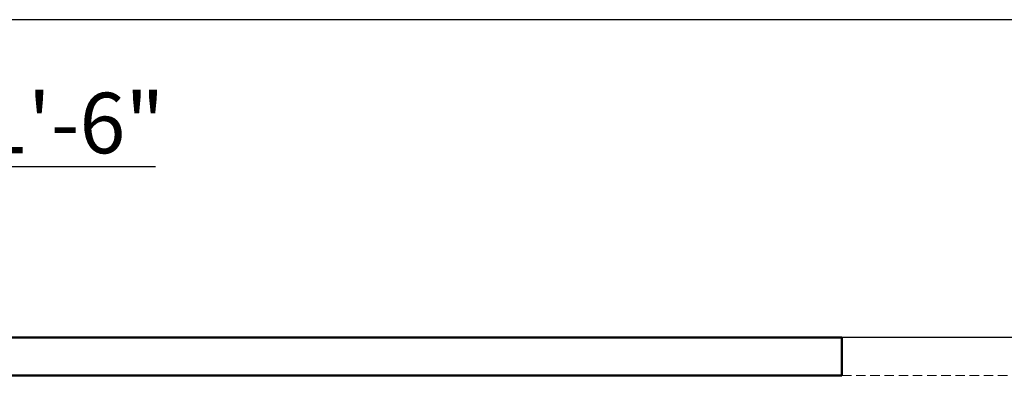
# Model space of a CAD drawing. Units: inches. Extents: x 1913 to 5309, y 1003 to 1733.
# Tile 4 of 23: x 2173 to 2303, y 1324 to 1371. Entities that reach past the tile are written whole.
import ezdxf

# ---------------------------------------------------------------- set-up
doc = ezdxf.new("R2010")
doc.units = ezdxf.units.IN
doc.linetypes.add('HIDDEN2', pattern=[0.1875, 0.125, -0.0625])
for name, color, linetype, lineweight in [('A-ANNO-DIMS', 2, 'Continuous', 18), ('A-WALL', 7, 'Continuous', 50), ('A-WALL-OVHD', 8, 'HIDDEN2', 18)]:
    doc.layers.add(name, color=color, linetype=linetype, lineweight=lineweight)
doc.styles.get("Standard").update_dxf_attribs({"font": 'arial.ttf'})
doc.dimstyles.new('ISO-25', dxfattribs={"dimtxt": 8, "dimasz": 2.5, "dimexe": 1.25, "dimexo": 0.625, "dimtad": 1, "dimdec": 1, "dimlunit": 3, "dimtxsty": 'Standard', "dimcen": 2.5, "dimclrd": 256, "dimclrt": 1, "dimadec": 0, "dimazin": 0, "dimtfac": 1, "dimtdec": 1, "dimtmove": 0, "dimatfit": 3, "dimfxl": 1, "dimarcsym": 0})

# ---------------------------------------------------------------- blocks, each defined once
blk = doc.blocks.new('*D88')
at = {"layer": 'A-ANNO-DIMS', "color": 0, "lineweight": -2, "transparency": 16777216}
for p, q in [((2148.37, 1356.34), (2148.37, 1350.31)), ((2166.37, 1356.34), (2166.37, 1350.31))]:
    blk.add_line(p, q, dxfattribs=at)
at = {"layer": 'A-ANNO-DIMS', "lineweight": -2, "transparency": 16777216}
for p, q in [((2150.87, 1351.56), (2163.87, 1351.56)), ((2166.37, 1351.56), (2190.64, 1351.56))]:
    blk.add_line(p, q, dxfattribs=at)
at = {"layer": 'A-ANNO-DIMS', "transparency": 16777216}
for points in [[(2150.87, 1351.98), (2150.87, 1351.15), (2148.37, 1351.56)], [(2163.87, 1351.98), (2163.87, 1351.15), (2166.37, 1351.56)]]:
    blk.add_solid(points, dxfattribs=at)
at = {"layer": 'Defpoints', "color": 0, "transparency": 16777216}
for p in [(2148.37, 1356.96), (2166.37, 1356.96), (2166.37, 1351.56)]:
    blk.add_point(p, dxfattribs=at)
at = {"layer": 'A-ANNO-DIMS', "color": 1, "transparency": 16777216, "insert": (2179.75, 1356.27), "char_height": 8, "attachment_point": 5}
blk.add_mtext('1\'-6"', dxfattribs=at)
blk = doc.blocks.new('*D102')
at = {"layer": 'A-ANNO-DIMS', "color": 0, "lineweight": -2, "transparency": 16777216}
for p, q in [((2412.75, 1370.96), (1922.12, 1370.96)), ((2412.75, 1328.96), (1922.12, 1328.96))]:
    blk.add_line(p, q, dxfattribs=at)
at = {"layer": 'A-ANNO-DIMS', "lineweight": -2, "transparency": 16777216}
blk.add_line((1923.37, 1331.46), (1923.37, 1368.46), dxfattribs=at)
at = {"layer": 'A-ANNO-DIMS', "transparency": 16777216}
for points in [[(1922.96, 1368.46), (1923.79, 1368.46), (1923.37, 1370.96)], [(1922.96, 1331.46), (1923.79, 1331.46), (1923.37, 1328.96)]]:
    blk.add_solid(points, dxfattribs=at)
at = {"layer": 'Defpoints', "color": 0, "transparency": 16777216}
for p in [(1923.37, 1370.96), (2413.37, 1370.96), (2413.37, 1328.96)]:
    blk.add_point(p, dxfattribs=at)
at = {"layer": 'A-ANNO-DIMS', "color": 1, "transparency": 16777216, "insert": (1918.66, 1349.96), "char_height": 8, "attachment_point": 5, "rotation": 90}
blk.add_mtext('3\'-6"', dxfattribs=at)

msp = doc.modelspace()

# ---------------------------------------------------------------- linework, layer by layer
at = {"layer": 'A-WALL'}
for p, q in [((2148.37, 1328.96), (2281.37, 1328.96)), ((2281.37, 1328.96), (2281.37, 1323.96)), ((2157.37, 1323.96), (2281.37, 1323.96))]:
    msp.add_line(p, q, dxfattribs=at)
at = {"layer": 'A-WALL-OVHD', "ltscale": 10}
for p, q in [((2281.37, 1328.96), (2341.37, 1328.96)), ((2281.37, 1323.96), (2341.37, 1323.96))]:
    msp.add_line(p, q, dxfattribs=at)

# ---------------------------------------------------------------- dimensions: what is measured, and where the dimension line sits
at = {"layer": 'A-ANNO-DIMS'}
dim = msp.add_linear_dim(base=(1923.37, 1370.96), p1=(2413.37, 1328.96), p2=(2413.37, 1370.96), angle=90, dimstyle='ISO-25', override={"dimdec": 1, "dimlfac": 1, "dimrnd": 0, "dimzin": 1, "dimdsep": 46, "dimlunit": 4, "dimfrac": 2}, dxfattribs=at)
dim.commit()
dim.dimension.update_dxf_attribs({"geometry": '*D102', "text_midpoint": (1918.66, 1349.96)})
dim = msp.add_linear_dim(base=(2166.37, 1351.56), p1=(2148.37, 1356.96), p2=(2166.37, 1356.96), dimstyle='ISO-25', override={"dimdec": 1, "dimrnd": 0, "dimzin": 1, "dimlunit": 4, "dimfrac": 2}, dxfattribs=at)
dim.commit()
dim.dimension.update_dxf_attribs({"geometry": '*D88', "text_midpoint": (2179.75, 1356.27)})

doc.saveas('drawing.dxf')
